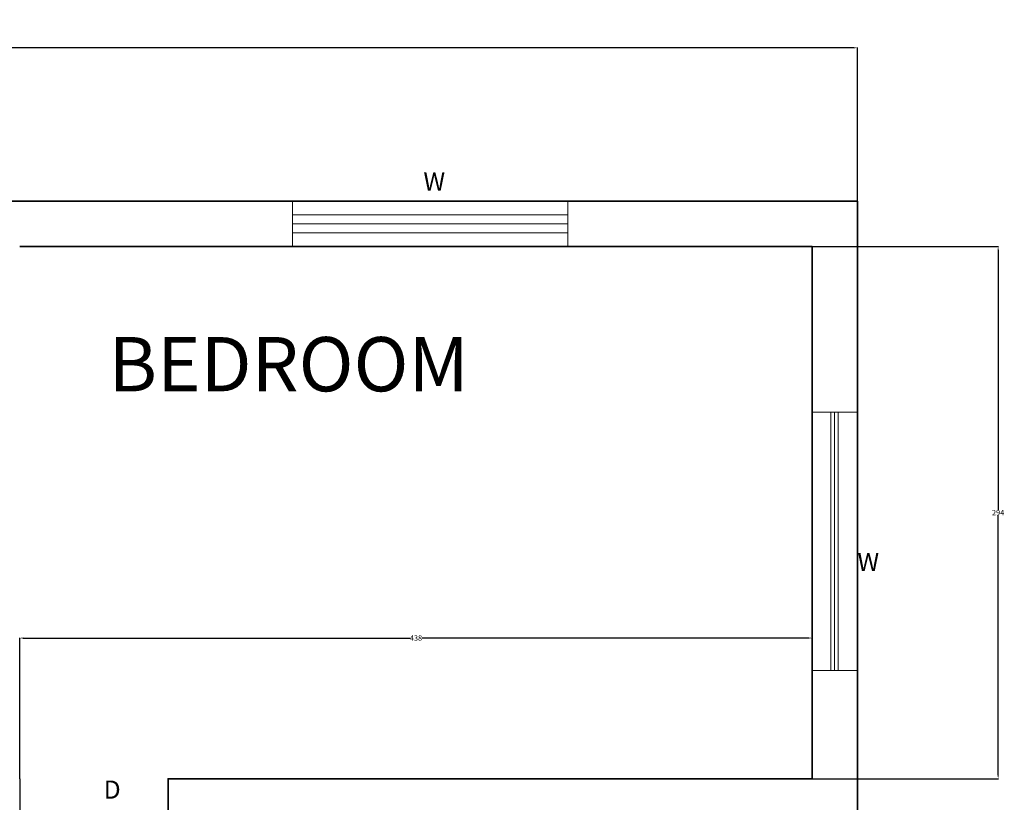
# Model space of a CAD drawing. Units: centimetres. Extents: x -121 to 3851, y -16 to 1180.
# Tile 9 of 16: x 958 to 1502, y 548 to 980. Entities that reach past the tile are written whole.
import ezdxf

# ---------------------------------------------------------------- set-up
doc = ezdxf.new("R2010")
doc.units = ezdxf.units.CM
doc.header["$MEASUREMENT"] = 0
for name, color, linetype, lineweight in [('A-ANNO-DIMS', 2, 'Continuous', 18), ('A-ANNO-IDEN', 3, 'Continuous', 13), ('A-AREA-IDEN', 3, 'Continuous', 18), ('A-GLAZ', 4, 'Continuous', 18), ('A-WALL', 7, 'Continuous', 35)]:
    doc.layers.add(name, color=color, linetype=linetype, lineweight=lineweight)
doc.styles.get("Standard").update_dxf_attribs({"font": 'arial.ttf'})
doc.dimstyles.get("Standard").update_dxf_attribs({"dimtxt": 3, "dimasz": 2, "dimexe": 0.18, "dimexo": 0.0625, "dimgap": 0.09, "dimtad": 0, "dimtih": 1, "dimtoh": 1, "dimdec": 0, "dimzin": 0, "dimdsep": 46, "dimtxsty": 'Standard', "dimcen": 0.09, "dimadec": 0, "dimazin": 0, "dimtfac": 1, "dimtdec": 0, "dimtofl": 0, "dimtmove": 0, "dimatfit": 3, "dimfxl": 1, "dimtolj": 1, "dimtzin": 0, "dimarcsym": 0})

# ---------------------------------------------------------------- blocks, each defined once
blk = doc.blocks.new('*D1')
at = {"layer": 'A-ANNO-DIMS', "color": 0, "lineweight": -2, "transparency": 16777216}
for p, q in [((65.04, 880.08), (65.04, 964.95)), ((67.04, 964.77), (699.58, 964.77)), ((1419.04, 964.77), (786.5, 964.77)), ((1421.04, 880.08), (1421.04, 964.95))]:
    blk.add_line(p, q, dxfattribs=at)
at = {"layer": 'A-ANNO-DIMS', "color": 0, "transparency": 16777216}
for points in [[(67.04, 965.1), (67.04, 964.43), (65.04, 964.77)], [(1419.04, 965.1), (1419.04, 964.43), (1421.04, 964.77)]]:
    blk.add_solid(points, dxfattribs=at)
at = {"layer": 'Defpoints', "color": 0, "transparency": 16777216}
for p in [(1421.04, 964.77), (65.04, 880.01), (1421.04, 880.01)]:
    blk.add_point(p, dxfattribs=at)
at = {"layer": 'A-ANNO-DIMS', "color": 0, "transparency": 16777216, "insert": (743.04, 964.77), "char_height": 3, "attachment_point": 5}
blk.add_mtext('\\A1;{\\H10x;1356}', dxfattribs=at)
blk = doc.blocks.new('WIN-152CM')
for p, q in [((0, 17.5), (152.19, 17.5)), ((0, 12.5), (152.19, 12.5)), ((0, 7.5), (152.19, 7.5))]:
    blk.add_line(p, q)
blk.add_lwpolyline([(0, 25), (152.19, 25), (152.19, 0), (0, 0)], close=True)
blk = doc.blocks.new('WIN-143CM')
for p, q in [((0, 14.5), (142.63, 14.5)), ((0, 12.5), (142.63, 12.5)), ((0, 10.5), (142.63, 10.5))]:
    blk.add_line(p, q)
blk.add_lwpolyline([(0, 25), (142.63, 25), (142.63, 0), (0, 0)], close=True)
blk = doc.blocks.new('*D39')
at = {"layer": 'A-ANNO-DIMS', "color": 0, "lineweight": -2, "transparency": 16777216}
for p, q in [((958.04, 561.08), (958.04, 638.94)), ((960.04, 638.76), (1173.57, 638.76)), ((1394.04, 638.76), (1180.51, 638.76)), ((1396.04, 561.08), (1396.04, 638.94))]:
    blk.add_line(p, q, dxfattribs=at)
at = {"layer": 'A-ANNO-DIMS', "color": 0, "transparency": 16777216}
for points in [[(960.04, 639.1), (960.04, 638.43), (958.04, 638.76)], [(1394.04, 639.1), (1394.04, 638.43), (1396.04, 638.76)]]:
    blk.add_solid(points, dxfattribs=at)
at = {"layer": 'Defpoints', "color": 0, "transparency": 16777216}
for p in [(1396.04, 638.76), (958.04, 561.01), (1396.04, 561.01)]:
    blk.add_point(p, dxfattribs=at)
at = {"layer": 'A-ANNO-DIMS', "color": 0, "transparency": 16777216, "insert": (1177.04, 638.76), "char_height": 3, "attachment_point": 5}
blk.add_mtext('\\A1;438', dxfattribs=at)
blk = doc.blocks.new('*D40')
at = {"layer": 'A-ANNO-DIMS', "color": 0, "lineweight": -2, "transparency": 16777216}
for p, q in [((1396.1, 855.01), (1498.97, 855.01)), ((1498.79, 853.01), (1498.79, 709.64)), ((1498.79, 563.01), (1498.79, 706.39)), ((1396.1, 561.01), (1498.97, 561.01))]:
    blk.add_line(p, q, dxfattribs=at)
at = {"layer": 'A-ANNO-DIMS', "color": 0, "transparency": 16777216}
for points in [[(1498.45, 853.01), (1499.12, 853.01), (1498.79, 855.01)], [(1498.45, 563.01), (1499.12, 563.01), (1498.79, 561.01)]]:
    blk.add_solid(points, dxfattribs=at)
at = {"layer": 'Defpoints', "color": 0, "transparency": 16777216}
for p in [(1396.04, 855.01), (1396.04, 561.01), (1498.79, 561.01)]:
    blk.add_point(p, dxfattribs=at)
at = {"layer": 'A-ANNO-DIMS', "color": 0, "transparency": 16777216, "insert": (1498.79, 708.01), "char_height": 3, "attachment_point": 5}
blk.add_mtext('\\A1;294', dxfattribs=at)
blk = doc.blocks.new('*D52')
at = {"layer": 'A-ANNO-DIMS', "color": 0, "lineweight": -2, "transparency": 16777216}
for p, q in [((958.04, 560.95), (958.04, 483.08)), ((1040.01, 560.95), (1040.01, 483.08)), ((960.04, 483.26), (993.87, 483.26)), ((1038.01, 483.26), (1004.18, 483.26))]:
    blk.add_line(p, q, dxfattribs=at)
at = {"layer": 'A-ANNO-DIMS', "color": 0, "transparency": 16777216}
for points in [[(960.04, 483.6), (960.04, 482.93), (958.04, 483.26)], [(1038.01, 483.6), (1038.01, 482.93), (1040.01, 483.26)]]:
    blk.add_solid(points, dxfattribs=at)
at = {"layer": 'Defpoints', "color": 0, "transparency": 16777216}
for p in [(958.04, 561.01), (1040.01, 561.01), (958.04, 483.26)]:
    blk.add_point(p, dxfattribs=at)
at = {"layer": 'A-ANNO-DIMS', "color": 0, "transparency": 16777216, "insert": (999.02, 483.26), "char_height": 3, "attachment_point": 5}
blk.add_mtext('\\A1;81.97', dxfattribs=at)

msp = doc.modelspace()

# ---------------------------------------------------------------- linework, layer by layer
at = {"layer": 'A-WALL'}
for p, q in [((390.0382, 880.0141), (1421.0382, 880.0141)), ((1421.0382, 880.0141), (1421.0382, 64.0141)), ((958.0382, 855.0141), (1396.0382, 855.0141)), ((1396.0382, 855.0141), (1396.0382, 561.0141)), ((1040.0075, 561.0141), (1396.0382, 561.0141))]:
    msp.add_line(p, q, dxfattribs=at)
msp.add_lwpolyline([(1060.101, 561.0141), (1040.0075, 561.0141), (1040.0075, 384.0141)], dxfattribs=at)

# ---------------------------------------------------------------- block references
at = {"layer": 'A-GLAZ'}
msp.add_blockref('WIN-152CM', (1108.7733, 855.014), dxfattribs=at)
at = {"layer": 'A-GLAZ', "rotation": 90.00000000000007}
msp.add_blockref('WIN-143CM', (1420.8472, 620.908), dxfattribs=at)

# ---------------------------------------------------------------- texts
at = {"layer": 'A-ANNO-IDEN', "char_height": 10, "attachment_point": 1}
for s, insert in [('W', (1181.1724, 895.9034)), ('W', (1421.0382, 685.8127)), ('D', (1004.4628, 560.0525))]:
    msp.add_mtext_dynamic_manual_height_columns(s, width=55.718495, gutter_width=1, heights=[0], dxfattribs=dict(at, insert=insert))
at = {"layer": 'A-AREA-IDEN', "insert": (1007.0546, 805.0234), "char_height": 30, "attachment_point": 1}
msp.add_mtext_dynamic_manual_height_columns('BEDROOM', width=248.976965, gutter_width=1, heights=[0], dxfattribs=at)

# ---------------------------------------------------------------- dimensions: what is measured, and where the dimension line sits
at = {"layer": 'A-ANNO-DIMS'}
dim = msp.add_linear_dim(base=(1421.0382, 964.7682), p1=(65.0382, 880.0141), p2=(1421.0382, 880.0141), text='{\\H10x;<>}', dimstyle='Standard', override={"dimclrd": 0, "dimclre": 0, "dimclrt": 0}, dxfattribs=at)
dim.commit()
dim.dimension.update_dxf_attribs({"geometry": '*D1', "text_midpoint": (743.0382, 964.7682)})
for base, p1, p2, angle, override, picture, middle in [((1498.7882, 561.0141), (1396.0382, 855.0141), (1396.0382, 561.0141), 90, {"dimdec": 0, "dimlfac": 1, "dimrnd": 0, "dimzin": 0, "dimdsep": 46, "dimlunit": 2}, '*D40', (1498.7882, 708.0141)), ((958.0382, 483.2641), (1040.0075, 561.0141), (958.0382, 561.0141), 180, {"dimdec": 2, "dimlfac": 1, "dimrnd": 0, "dimzin": 0, "dimdsep": 46, "dimlunit": 2}, '*D52', (999.0228, 483.2641))]:
    dim = msp.add_linear_dim(base=base, p1=p1, p2=p2, angle=angle, dimstyle='Standard', override=override, dxfattribs=at)
    dim.commit()
    dim.dimension.update_dxf_attribs({"geometry": picture, "text_midpoint": middle})
dim = msp.add_linear_dim(base=(1396.0382, 638.7641), p1=(958.0382, 561.0141), p2=(1396.0382, 561.0141), dimstyle='Standard', override={"dimdec": 0, "dimlfac": 1, "dimrnd": 0, "dimzin": 0, "dimdsep": 46, "dimlunit": 2}, dxfattribs=at)
dim.commit()
dim.dimension.update_dxf_attribs({"geometry": '*D39', "text_midpoint": (1177.0382, 638.7641)})

doc.saveas('drawing.dxf')
